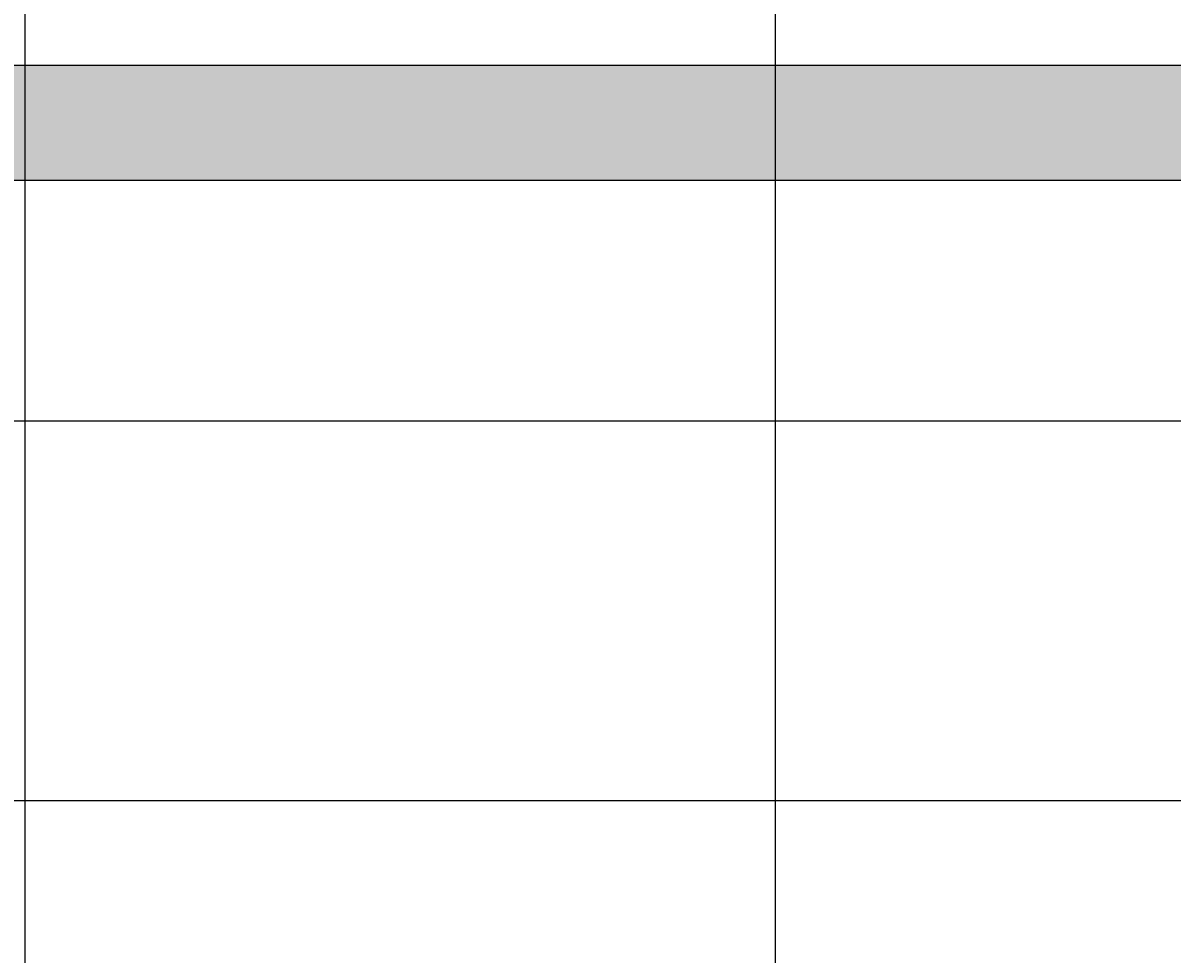
# Model space of a CAD drawing. Units: millimetres. Extents: x -11 to 280, y -4 to 208.
# Tile 45 of 55: x 151 to 186, y 128 to 157. Entities that reach past the tile are written whole.
import ezdxf

# ---------------------------------------------------------------- set-up
doc = ezdxf.new("R2010")
doc.units = ezdxf.units.MM
doc.layers.add('M-DIMS', color=2, linetype='Continuous', lineweight=18)
doc.layers.add('M-HYDR-SUCT', color=7, linetype='Continuous', lineweight=25)
doc.layers.add('M-HYDR-SUCT-PATT', color=221, linetype='Continuous', lineweight=13, true_color=0xff7fdf)
doc.styles.get("Standard").update_dxf_attribs({"font": 'arial.ttf'})
doc.dimstyles.get("Standard").update_dxf_attribs({"dimtxt": 0.18, "dimasz": 0.18, "dimexe": 0.18, "dimexo": 0.0625, "dimgap": 0.09, "dimtad": 0, "dimtih": 1, "dimtoh": 1, "dimdec": 4, "dimzin": 0, "dimdsep": 46, "dimtxsty": 'Standard', "dimcen": 0.09, "dimadec": 0, "dimazin": 0, "dimtfac": 1, "dimtdec": 4, "dimtofl": 0, "dimtmove": 0, "dimatfit": 3, "dimfxl": 1, "dimtolj": 1, "dimtzin": 0, "dimarcsym": 0})

# ---------------------------------------------------------------- blocks, each defined once
blk = doc.blocks.new('*D5')
at = {"layer": 'Defpoints', "color": 0, "transparency": 16777216}
for p in [(24.759, 192.645), (-10.087, 11.435), (261.686, 11.435)]:
    blk.add_point(p, dxfattribs=at)
at = {"layer": 'M-DIMS', "color": 0, "lineweight": -2, "transparency": 16777216}
for p, q in [((24.696, 192.645), (-10.267, 192.645)), ((-10.087, 192.465), (-10.087, 102.222)), ((-10.087, 11.615), (-10.087, 101.858)), ((261.624, 11.435), (-10.267, 11.435))]:
    blk.add_line(p, q, dxfattribs=at)
at = {"layer": 'M-DIMS', "color": 0, "transparency": 16777216}
for points in [[(-10.117, 192.465), (-10.057, 192.465), (-10.087, 192.645)], [(-10.117, 11.615), (-10.057, 11.615), (-10.087, 11.435)]]:
    blk.add_solid(points, dxfattribs=at)
at = {"layer": 'M-DIMS', "color": 0, "transparency": 16777216, "insert": (-10.087, 102.04), "char_height": 0.18, "attachment_point": 5}
blk.add_mtext('\\A1;181.2', dxfattribs=at)
blk = doc.blocks.new('*D12')
at = {"layer": 'Defpoints', "color": 0, "transparency": 16777216}
for p in [(173.804, 207.495), (118.514, 96.485), (173.804, 89.387)]:
    blk.add_point(p, dxfattribs=at)
at = {"layer": 'M-DIMS', "color": 0, "lineweight": -2, "transparency": 16777216}
for p, q in [((118.514, 96.547), (118.514, 207.675)), ((118.694, 207.495), (145.765, 207.495)), ((173.624, 207.495), (146.553, 207.495)), ((173.804, 89.45), (173.804, 207.675))]:
    blk.add_line(p, q, dxfattribs=at)
at = {"layer": 'M-DIMS', "color": 0, "transparency": 16777216}
for points in [[(118.694, 207.525), (118.694, 207.465), (118.514, 207.495)], [(173.624, 207.525), (173.624, 207.465), (173.804, 207.495)]]:
    blk.add_solid(points, dxfattribs=at)
at = {"layer": 'M-DIMS', "color": 0, "transparency": 16777216, "insert": (146.159, 207.495), "char_height": 0.18, "attachment_point": 5}
blk.add_mtext('\\A1;55.29', dxfattribs=at)
blk = doc.blocks.new('*D14')
at = {"layer": 'Defpoints', "color": 0, "transparency": 16777216}
for p in [(-10.087, 144.661), (205.531, 144.661), (226.511, 133.123)]:
    blk.add_point(p, dxfattribs=at)
at = {"layer": 'M-DIMS', "color": 0, "lineweight": -2, "transparency": 16777216}
for p, q in [((205.469, 144.661), (-10.267, 144.661)), ((-10.087, 144.481), (-10.087, 139.074)), ((-10.087, 133.303), (-10.087, 138.71)), ((226.448, 133.123), (-10.267, 133.123))]:
    blk.add_line(p, q, dxfattribs=at)
at = {"layer": 'M-DIMS', "color": 0, "transparency": 16777216}
for points in [[(-10.117, 144.481), (-10.057, 144.481), (-10.087, 144.661)], [(-10.117, 133.303), (-10.057, 133.303), (-10.087, 133.123)]]:
    blk.add_solid(points, dxfattribs=at)
at = {"layer": 'M-DIMS', "color": 0, "transparency": 16777216, "insert": (-10.087, 138.892), "char_height": 0.18, "attachment_point": 5}
blk.add_mtext('\\A1;11.538', dxfattribs=at)
blk = doc.blocks.new('*D18')
at = {"layer": 'Defpoints', "color": 0, "transparency": 16777216}
for p in [(173.804, 207.495), (173.804, 65.064), (151.022, 43.599)]:
    blk.add_point(p, dxfattribs=at)
at = {"layer": 'M-DIMS', "color": 0, "lineweight": -2, "transparency": 16777216}
for p, q in [((151.022, 43.662), (151.022, 207.675)), ((151.202, 207.495), (162.017, 207.495)), ((173.624, 207.495), (162.808, 207.495)), ((173.804, 65.126), (173.804, 207.675))]:
    blk.add_line(p, q, dxfattribs=at)
at = {"layer": 'M-DIMS', "color": 0, "transparency": 16777216}
for points in [[(151.202, 207.525), (151.202, 207.465), (151.022, 207.495)], [(173.624, 207.525), (173.624, 207.465), (173.804, 207.495)]]:
    blk.add_solid(points, dxfattribs=at)
at = {"layer": 'M-DIMS', "color": 0, "transparency": 16777216, "insert": (162.413, 207.495), "char_height": 0.18, "attachment_point": 5}
blk.add_mtext('\\A1;22.78', dxfattribs=at)
blk = doc.blocks.new('*D20')
at = {"layer": 'Defpoints', "color": 0, "transparency": 16777216}
for p in [(231.68, 207.495), (151.022, 43.599), (231.68, 43.599)]:
    blk.add_point(p, dxfattribs=at)
at = {"layer": 'M-DIMS', "color": 0, "lineweight": -2, "transparency": 16777216}
for p, q in [((151.022, 43.662), (151.022, 207.675)), ((151.202, 207.495), (190.957, 207.495)), ((231.5, 207.495), (191.745, 207.495)), ((231.68, 43.662), (231.68, 207.675))]:
    blk.add_line(p, q, dxfattribs=at)
at = {"layer": 'M-DIMS', "color": 0, "transparency": 16777216}
for points in [[(151.202, 207.525), (151.202, 207.465), (151.022, 207.495)], [(231.5, 207.525), (231.5, 207.465), (231.68, 207.495)]]:
    blk.add_solid(points, dxfattribs=at)
at = {"layer": 'M-DIMS', "color": 0, "transparency": 16777216, "insert": (191.351, 207.495), "char_height": 0.18, "attachment_point": 5}
blk.add_mtext('\\A1;80.66', dxfattribs=at)

msp = doc.modelspace()

# ---------------------------------------------------------------- hatches: boundary and pattern name
at = {"layer": 'M-HYDR-SUCT-PATT'}
h = msp.add_hatch(color=256, dxfattribs=at)
h.set_gradient(color1=(255, 127, 223), color2=(255, 127, 223), tint=1, name='INVCYLINDER')
h.paths.add_polyline_path([(91.3629, 155.4768), (91.3629, 132.4768), (58.3629, 132.4768), (58.3629, 153.9768), (54.8629, 153.9768), (54.8629, 128.9768), (94.8629, 128.9768), (94.8629, 151.9768), (205.5315, 151.9768), (205.5315, 155.4768)])
h.paths.add_polyline_path([(91.3, 114.9452, 1), (78.8273, 114.9452), (78.8273, 108.8141), (42.6453, 108.8141), (42.6453, 153.9768), (39.1453, 153.9768), (39.1453, 105.3141), (78.8273, 105.3141), (78.8273, 98.1491, 1), (91.3, 98.1491), (91.3, 105.3141), (95.5776, 105.3141), (95.5776, 108.8141), (91.3, 108.8141)])
h.paths.add_polyline_path([(228.7, 138.4081), (232.2, 138.4081), (232.2, 144.6609), (228.7, 144.6609)])
h.paths.add_polyline_path([(253.1005, 151.9768, 1), (253.1005, 155.4768), (252.6001, 155.4768), (253.5249, 153.991, -0.1401047), (253.6005, 153.7268, -0.7542249), (252.676, 153.4626), (251.4221, 155.4768), (236.9353, 155.4768), (236.9353, 151.9768)])
h.paths.add_polyline_path([(30.8182, 40.7626), (30.8182, 36.7626), (60.8182, 36.7626), (60.8182, 40.7626)])

# ---------------------------------------------------------------- linework, layer by layer
at = {"layer": 'M-HYDR-SUCT'}
for points in [[(58.3629, 153.9768), (58.3629, 132.4768), (91.3629, 132.4768), (91.3629, 155.4768), (205.5315, 155.4768)], [(54.8629, 153.9768), (54.8629, 128.9768), (94.8629, 128.9768), (94.8629, 151.9768), (205.5315, 151.9768)]]:
    msp.add_lwpolyline(points, dxfattribs=at)

# ---------------------------------------------------------------- dimensions: what is measured, and where the dimension line sits
at = {"layer": 'M-DIMS'}
for base, p1, p2, picture, middle in [((173.8038, 207.495), (118.5137, 96.4849), (173.8038, 89.3873), '*D12', (146.1587, 207.495)), ((173.8038, 207.495), (151.0217, 43.5991), (173.8038, 65.0638), '*D18', (162.4127, 207.495)), ((231.6803, 207.495), (151.0217, 43.5991), (231.6803, 43.5991), '*D20', (191.351, 207.495))]:
    dim = msp.add_linear_dim(base=base, p1=p1, p2=p2, dimstyle='Standard', override={"dimdec": 2, "dimlfac": 1, "dimrnd": 0, "dimzin": 0, "dimdsep": 46, "dimlunit": 2}, dxfattribs=at)
    dim.commit()
    dim.dimension.update_dxf_attribs({"geometry": picture, "text_midpoint": middle})
for base, p1, p2, override, picture, middle in [((-10.0865, 11.4346), (24.7588, 192.645), (261.6863, 11.4346), {"dimdec": 1, "dimlfac": 1, "dimrnd": 0, "dimzin": 0, "dimdsep": 46, "dimlunit": 2}, '*D5', (-10.0865, 102.0398)), ((-10.0865, 144.6609), (226.5106, 133.1228), (205.5315, 144.6609), {"dimdec": 3, "dimlfac": 1, "dimrnd": 0, "dimzin": 0, "dimdsep": 46, "dimlunit": 2}, '*D14', (-10.0865, 138.8918))]:
    dim = msp.add_linear_dim(base=base, p1=p1, p2=p2, angle=90, dimstyle='Standard', override=override, dxfattribs=at)
    dim.commit()
    dim.dimension.update_dxf_attribs({"geometry": picture, "text_midpoint": middle})

doc.saveas('drawing.dxf')
